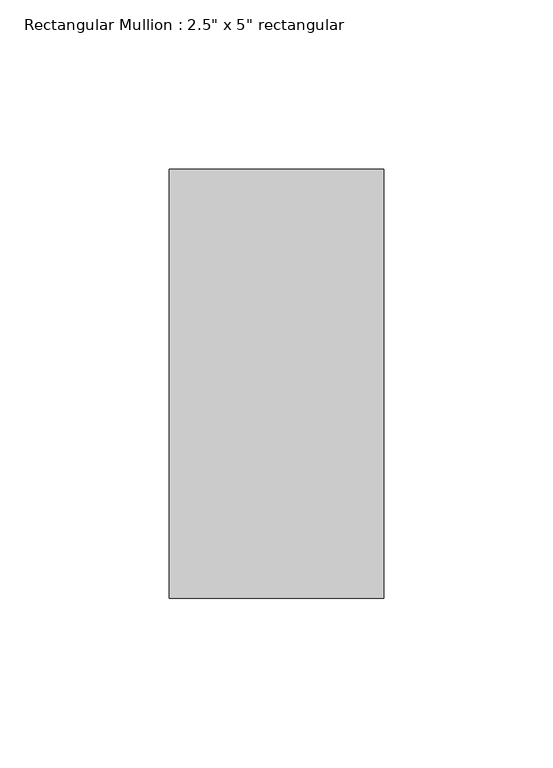
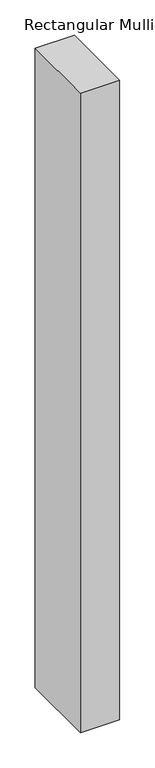
"""IFC4 building model written with IfcOpenShell, lengths in millimetres: member geometry."""

from ifc_helpers import new_model, si_unit, frame, origin, place, context, project, spatial, polyline, outline, extrude, source, transform, mapped, element, save


def member_3972cc06(model_context):
    return source(origin(), model_context, "Body", "SweptSolid", [
        extrude(outline(polyline([(0.0, 63.5), (0.0, -63.5), (-63.5, -63.5), (-63.5, 63.5), (0.0, 63.5)])), frame((0.0, 0.0, -1099.5770399), z_axis=(0.0, 0.0, 1.0), x_axis=(1.0, 0.0, 0.0)), (0.0, 0.0, 1.0), 1099.5770399),
    ])


if __name__ == "__main__":
    model = new_model("IFC4")
    model_context = context("Model", 3, world=origin())
    ifc_project = project(units=[si_unit("LENGTHUNIT", "METRE", prefix="MILLI")], contexts=[model_context])
    site = spatial("IfcSite", under=ifc_project)
    building = spatial("IfcBuilding", under=site)
    placement = place(None, origin())
    member_shape = member_3972cc06(model_context)
    element("IfcMember", 1, ObjectType="Rectangular Mullion : 2.5\" x 5\" rectangular", at=placement, inside=building, context=model_context, shape_type="MappedRepresentation", body=[
        mapped(member_shape, transform((0.0, 0.0, 0.0), x_axis=(1.0, 0.0, 0.0), y_axis=(0.0, 1.0, 0.0), z_axis=(0.0, 0.0, 1.0))),
    ])
    save(model, "model.ifc")

# Revit data of these elements
# Type "Rectangular Mullion : 2.5\" x 5\" rectangular"
#   built-in parameter 1007304 = 0.416667 (stored number, unit not read)
#   built-in parameter 1007301 = 0.104167 (stored number, unit not read)
#   built-in parameter 1007300 = 0.104167 (stored number, unit not read)
# Element 1 (IfcMember, "Rectangular Mullion : 2.5\" x 5\" rectangular")
#   Materials on its faces: "Aluminum"
# Materials
#   "Aluminum": class "Metal", colour RGB 247 247 247, transparency 0, Description = "Aluminum 6061", Cost = 0
